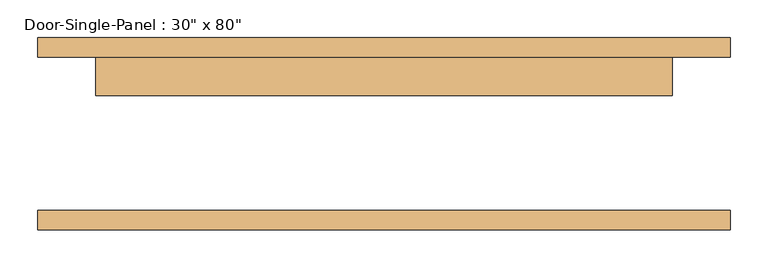
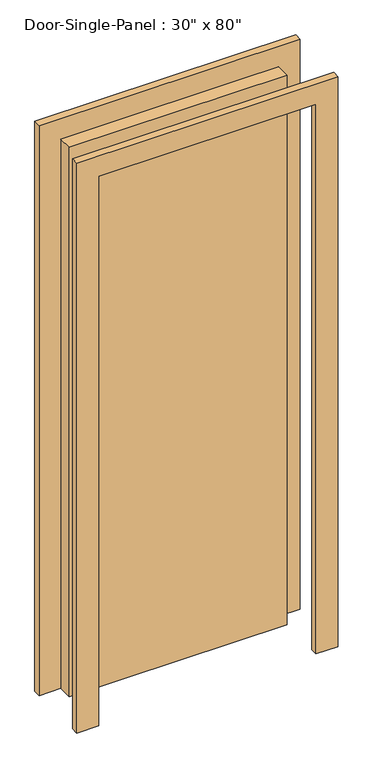
"""IFC4 building model written with IfcOpenShell, lengths in millimetres: door geometry."""

from ifc_helpers import new_model, si_unit, frame, origin, origin_with_axes, place, context, project, spatial, polyline, outline, extrude, source, transform, mapped, element, save


def door_1a782ffc(model_context):
    return source(origin(), model_context, "Body", "SweptSolid", [
        extrude(outline(polyline([(381.0, 50.8), (-381.0, 50.8), (-381.0, 101.6), (381.0, 101.6), (381.0, 50.8)])), origin_with_axes(), (0.0, 0.0, 1.0), 2032.0),
        extrude(outline(polyline([(2108.2, -457.2), (0.0, -457.2), (0.0, -381.0), (2032.0, -381.0), (2032.0, 381.0), (0.0, 381.0), (0.0, 457.2), (2108.2, 457.2), (2108.2, -457.2)])), frame((0.0, 101.6, 0.0), z_axis=(0.0, 1.0, 0.0), x_axis=(0.0, 0.0, 1.0)), (0.0, 0.0, 1.0), 25.4),
        extrude(outline(polyline([(2108.2, 457.2), (2108.2, -457.2), (0.0, -457.2), (0.0, -381.0), (2032.0, -381.0), (2032.0, 381.0), (0.0, 381.0), (0.0, 457.2), (2108.2, 457.2)])), frame((0.0, -127.0, 0.0), z_axis=(0.0, 1.0, 0.0), x_axis=(0.0, 0.0, 1.0)), (0.0, 0.0, 1.0), 25.4),
    ])


if __name__ == "__main__":
    model = new_model("IFC4")
    model_context = context("Model", 3, world=origin())
    ifc_project = project(units=[si_unit("LENGTHUNIT", "METRE", prefix="MILLI")], contexts=[model_context])
    site = spatial("IfcSite", under=ifc_project)
    building = spatial("IfcBuilding", under=site)
    placement = place(None, origin())
    door_shape = door_1a782ffc(model_context)
    element("IfcDoor", 1, ObjectType="Door-Single-Panel : 30\" x 80\"", at=placement, inside=building, context=model_context, shape_type="MappedRepresentation", body=[
        mapped(door_shape, transform((0.0, 0.0, 0.0), x_axis=(1.0, 0.0, 0.0), y_axis=(0.0, 1.0, 0.0), z_axis=(0.0, 0.0, 1.0))),
    ])
    save(model, "model.ifc")

# Revit data of these elements
# Type "Door-Single-Panel : 30\" x 80\""
#   Type Mark = "10"
#   Construction Type Id = "DOOR"
#   Assembly Code = "C1020300"
#   Analytic Construction = "Wooden"
#   Thickness = 0' - 2"
#   Thermal Resistance (R) = 2.5876 (h·ft²·°F)/BTU
#   Swing Angle [instance default] = 90.00°
#   Heat Transfer Coefficient (U) = 0.3865 BTU/(h·ft²·°F)
#   Height = 6' - 8"
#   Trim Projection Ext = 0' - 1"
#   Trim Projection Int = 0' - 1"
#   Trim Width = 0' - 3"
#   Width = 2' - 6"
#   Define Thermal Properties by = 1
#   Panel Material = Wood - Birch - Solid Stained Light Low Gloss
#   Trim Material = Paint - Sienna
#   Visual Light Transmittance = 0
#   Solar Heat Gain Coefficient = 0
#   Function = (empty or 0)
#   Wall Closure = (empty or 0)
# Element 1 (IfcDoor, "Door-Single-Panel : 30\" x 80\"")
#   Materials on its faces: "Paint - Sienna", "Wood - Birch - Solid Stained Light Low Gloss"
# Materials
#   "Wood - Birch - Solid Stained Light Low Gloss": class "Wood", colour RGB 210 159 95, transparency 0, Cost = 0
#   "Paint - Sienna": colour RGB 118 70 51, transparency 0, Cost = 0
